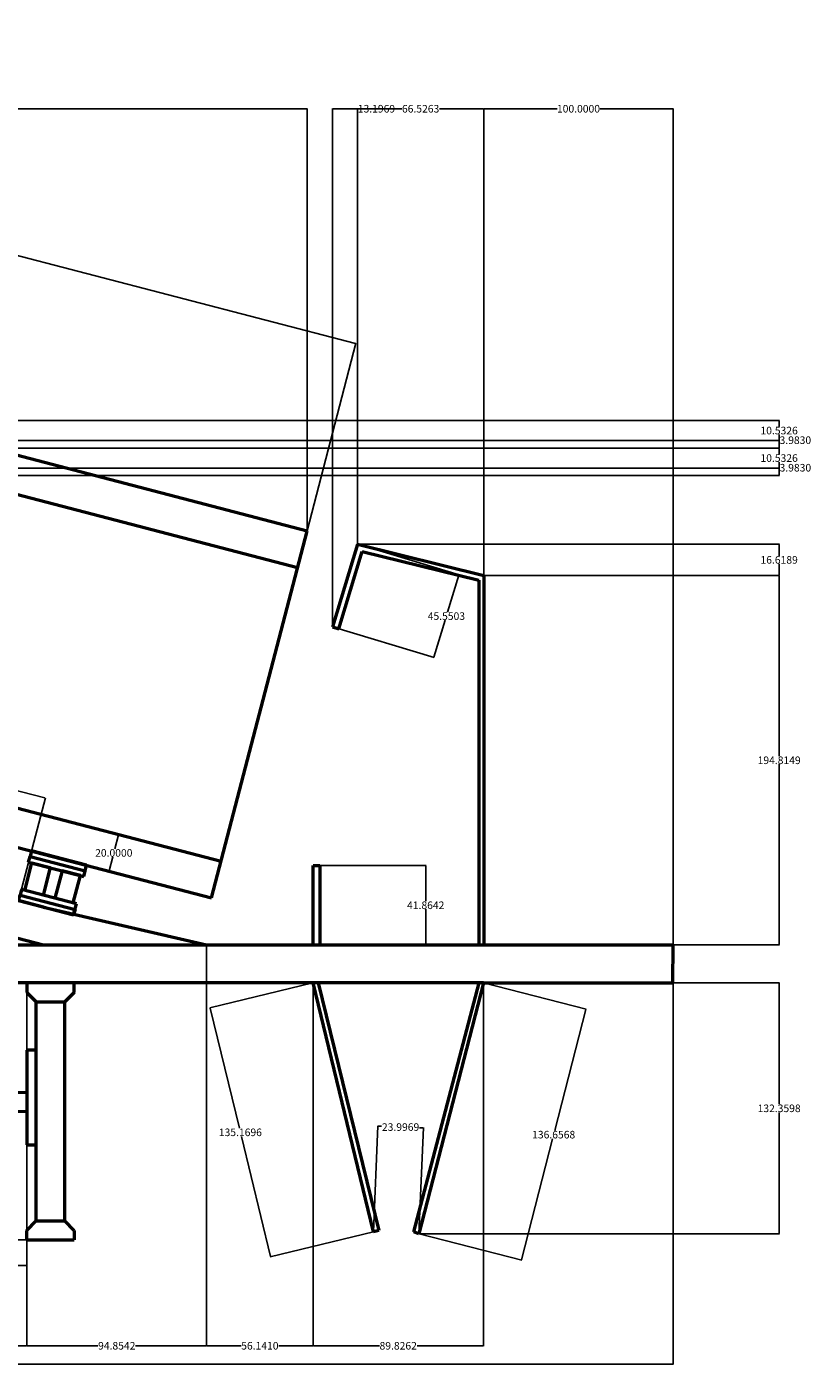
# Model space of a CAD drawing. Units: millimetres. Extents: x -54 to 1187, y -193 to 515.
# Tile 3 of 3: x 773 to 1187, y -193 to 515. Entities that reach past the tile are written whole.
import ezdxf

# ---------------------------------------------------------------- set-up
doc = ezdxf.new("R2010")
doc.units = ezdxf.units.MM
doc.header["$MEASUREMENT"] = 0
doc.layers.add('M-DIMS', color=2, linetype='Continuous', lineweight=25)
doc.layers.add('M-OUTL', color=7, linetype='Continuous', lineweight=50)
doc.styles.get("Standard").update_dxf_attribs({"font": 'arial.ttf'})
doc.dimstyles.get("Standard").update_dxf_attribs({"dimtxt": 4, "dimasz": 0.18, "dimexe": 0.18, "dimexo": 0.0625, "dimgap": 0.09, "dimtad": 0, "dimtih": 1, "dimtoh": 1, "dimdec": 4, "dimzin": 0, "dimdsep": 46, "dimtxsty": 'Standard', "dimcen": 0.09, "dimclrd": 3, "dimclre": 3, "dimclrt": 1, "dimadec": 0, "dimazin": 0, "dimtfac": 1, "dimtdec": 4, "dimtofl": 0, "dimtmove": 0, "dimatfit": 3, "dimfxl": 1, "dimtolj": 1, "dimtzin": 0, "dimarcsym": 0})

# ---------------------------------------------------------------- blocks, each defined once
blk = doc.blocks.new('*D1')
at = {"layer": 'Defpoints', "color": 0, "transparency": 16777216}
for p in [(13.68, 20.33), (1113.76, 20.33), (1113.76, -190.81)]:
    blk.add_point(p, dxfattribs=at)
at = {"layer": 'M-DIMS', "color": 0, "lineweight": -2, "transparency": 16777216}
for p, q in [((13.68, 20.27), (13.68, -190.99)), ((1113.76, 20.27), (1113.76, -190.99)), ((13.86, -190.81), (550.84, -190.81)), ((1113.58, -190.81), (576.6, -190.81))]:
    blk.add_line(p, q, dxfattribs=at)
at = {"layer": 'M-DIMS', "color": 0, "transparency": 16777216}
for points in [[(13.86, -190.78), (13.86, -190.84), (13.68, -190.81)], [(1113.58, -190.78), (1113.58, -190.84), (1113.76, -190.81)]]:
    blk.add_solid(points, dxfattribs=at)
at = {"layer": 'M-DIMS', "color": 0, "transparency": 16777216, "insert": (563.72, -190.81), "char_height": 4, "attachment_point": 5}
blk.add_mtext('\\A1;1100.0835', dxfattribs=at)
blk = doc.blocks.new('*D4')
at = {"layer": 'Defpoints', "color": 0, "transparency": 16777216}
for p in [(643.49, -51.86), (772.88, -51.86), (772.88, -138.82)]:
    blk.add_point(p, dxfattribs=at)
at = {"layer": 'M-DIMS', "color": 0, "lineweight": -2, "transparency": 16777216}
for p, q in [((643.49, -51.92), (643.49, -139)), ((772.88, -51.92), (772.88, -139)), ((643.67, -138.82), (696.87, -138.82)), ((772.7, -138.82), (719.5, -138.82))]:
    blk.add_line(p, q, dxfattribs=at)
at = {"layer": 'M-DIMS', "color": 0, "transparency": 16777216}
for points in [[(643.67, -138.79), (643.67, -138.85), (643.49, -138.82)], [(772.7, -138.79), (772.7, -138.85), (772.88, -138.82)]]:
    blk.add_solid(points, dxfattribs=at)
at = {"layer": 'M-DIMS', "color": 0, "transparency": 16777216, "insert": (708.19, -138.82), "char_height": 4, "attachment_point": 5}
blk.add_mtext('\\A1;129.3903', dxfattribs=at)
blk = doc.blocks.new('*D6')
at = {"layer": 'Defpoints', "color": 0, "transparency": 16777216}
for p in [(279.97, 415.58), (946.42, 347.55), (920.66, 248.68)]:
    blk.add_point(p, dxfattribs=at)
at = {"layer": 'M-DIMS', "color": 0, "lineweight": -2, "transparency": 16777216}
for p, q in [((279.99, 415.64), (305.78, 514.63)), ((305.91, 514.41), (617.89, 433.14)), ((946.25, 347.6), (634.26, 428.87)), ((920.68, 248.74), (946.47, 347.73))]:
    blk.add_line(p, q, dxfattribs=at)
at = {"layer": 'M-DIMS', "color": 0, "transparency": 16777216}
for points in [[(305.91, 514.44), (305.9, 514.38), (305.73, 514.46)], [(946.26, 347.63), (946.24, 347.57), (946.42, 347.55)]]:
    blk.add_solid(points, dxfattribs=at)
at = {"layer": 'M-DIMS', "color": 0, "transparency": 16777216, "insert": (626.08, 431.01), "char_height": 4, "attachment_point": 5}
blk.add_mtext('\\A1;662.0724', dxfattribs=at)
blk = doc.blocks.new('ROLLER-BEARING-UNIT')
for p, q in [((5.29, 27.88), (6.05, 30.79)), ((6.81, 33.69), (6.05, 30.79)), ((6.05, 30.79), (35.08, 23.23)), ((35.84, 26.13), (6.81, 33.69)), ((3.24, 12.92), (7.02, 27.44)), ((5.29, 27.88), (34.33, 20.32)), ((7.02, 27.44), (16.7, 24.91)), ((16.7, 24.91), (12.91, 10.4)), ((22.91, 23.3), (19.12, 8.78)), ((32.58, 20.78), (22.91, 23.3)), ((34.33, 20.32), (35.84, 26.13)), ((28.8, 6.26), (32.58, 20.78)), ((0, 7.56), (0.76, 10.47)), ((0, 7.56), (29.03, 0)), ((1.51, 13.37), (0.76, 10.47)), ((0.76, 10.47), (29.79, 2.9)), ((30.54, 5.81), (1.51, 13.37)), ((30.54, 5.81), (28.8, 6.26)), ((29.03, 0), (30.54, 5.81)), ((29.79, 2.9), (29.03, 0))]:
    blk.add_line(p, q)
blk = doc.blocks.new('FLANGE-PLATE')
for p, q in [((0, 50), (0, 0)), ((5, 50), (0, 50)), ((5, 0), (5, 50)), ((0, 0), (5, 0))]:
    blk.add_line(p, q)
blk = doc.blocks.new('*D13')
at = {"layer": 'Defpoints', "color": 0, "transparency": 16777216}
for p in [(-42.17, 415.58), (279.97, 415.58), (772.86, -125.25)]:
    blk.add_point(p, dxfattribs=at)
at = {"layer": 'M-DIMS', "color": 3, "lineweight": -2, "transparency": 16777216}
for p, q in [((279.91, 415.58), (-42.35, 415.58)), ((-42.17, 415.4), (-42.17, 147.3)), ((-42.17, -125.07), (-42.17, 143.03)), ((772.79, -125.25), (-42.35, -125.25))]:
    blk.add_line(p, q, dxfattribs=at)
at = {"layer": 'M-DIMS', "color": 3, "transparency": 16777216}
for points in [[(-42.2, 415.4), (-42.14, 415.4), (-42.17, 415.58)], [(-42.2, -125.07), (-42.14, -125.07), (-42.17, -125.25)]]:
    blk.add_solid(points, dxfattribs=at)
at = {"layer": 'M-DIMS', "color": 1, "transparency": 16777216, "insert": (-42.17, 145.16), "char_height": 4, "attachment_point": 5}
blk.add_mtext('\\A1;540.8329', dxfattribs=at)
blk = doc.blocks.new('*D18')
at = {"layer": 'Defpoints', "color": 0, "transparency": 16777216}
for p in [(618.49, 10.33), (772.86, 10.33), (772.86, -181.1)]:
    blk.add_point(p, dxfattribs=at)
at = {"layer": 'M-DIMS', "color": 3, "lineweight": -2, "transparency": 16777216}
for p, q in [((618.49, 10.27), (618.49, -181.28)), ((772.86, 10.27), (772.86, -181.28)), ((618.67, -181.1), (684.38, -181.1)), ((772.68, -181.1), (706.97, -181.1))]:
    blk.add_line(p, q, dxfattribs=at)
at = {"layer": 'M-DIMS', "color": 3, "transparency": 16777216}
for points in [[(618.67, -181.07), (618.67, -181.13), (618.49, -181.1)], [(772.68, -181.07), (772.68, -181.13), (772.86, -181.1)]]:
    blk.add_solid(points, dxfattribs=at)
at = {"layer": 'M-DIMS', "color": 1, "transparency": 16777216, "insert": (695.67, -181.1), "char_height": 4, "attachment_point": 5}
blk.add_mtext('\\A1;154.3662', dxfattribs=at)
blk = doc.blocks.new('*D19')
at = {"layer": 'Defpoints', "color": 0, "transparency": 16777216}
for p in [(867.71, 30.33), (772.86, 10.33), (867.71, -181.1)]:
    blk.add_point(p, dxfattribs=at)
at = {"layer": 'M-DIMS', "color": 3, "lineweight": -2, "transparency": 16777216}
for p, q in [((867.71, 30.27), (867.71, -181.28)), ((772.86, 10.27), (772.86, -181.28)), ((773.04, -181.1), (810.36, -181.1)), ((867.53, -181.1), (830.21, -181.1))]:
    blk.add_line(p, q, dxfattribs=at)
at = {"layer": 'M-DIMS', "color": 3, "transparency": 16777216}
for points in [[(773.04, -181.07), (773.04, -181.13), (772.86, -181.1)], [(867.53, -181.07), (867.53, -181.13), (867.71, -181.1)]]:
    blk.add_solid(points, dxfattribs=at)
at = {"layer": 'M-DIMS', "color": 1, "transparency": 16777216, "insert": (820.28, -181.1), "char_height": 4, "attachment_point": 5}
blk.add_mtext('\\A1;94.8542', dxfattribs=at)
blk = doc.blocks.new('*D20')
at = {"layer": 'Defpoints', "color": 0, "transparency": 16777216}
for p in [(867.71, 30.33), (923.85, 10.33), (923.85, -181.1)]:
    blk.add_point(p, dxfattribs=at)
at = {"layer": 'M-DIMS', "color": 3, "lineweight": -2, "transparency": 16777216}
for p, q in [((867.71, 30.27), (867.71, -181.28)), ((923.85, 10.27), (923.85, -181.28)), ((867.89, -181.1), (885.84, -181.1)), ((923.67, -181.1), (905.72, -181.1))]:
    blk.add_line(p, q, dxfattribs=at)
at = {"layer": 'M-DIMS', "color": 3, "transparency": 16777216}
for points in [[(867.89, -181.07), (867.89, -181.13), (867.71, -181.1)], [(923.67, -181.07), (923.67, -181.13), (923.85, -181.1)]]:
    blk.add_solid(points, dxfattribs=at)
at = {"layer": 'M-DIMS', "color": 1, "transparency": 16777216, "insert": (895.78, -181.1), "char_height": 4, "attachment_point": 5}
blk.add_mtext('\\A1;56.1410', dxfattribs=at)
blk = doc.blocks.new('*D21')
at = {"layer": 'Defpoints', "color": 0, "transparency": 16777216}
for p in [(923.85, 10.33), (1013.68, 10.33), (1013.68, -181.1)]:
    blk.add_point(p, dxfattribs=at)
at = {"layer": 'M-DIMS', "color": 3, "lineweight": -2, "transparency": 16777216}
for p, q in [((923.85, 10.27), (923.85, -181.28)), ((1013.68, 10.27), (1013.68, -181.28)), ((924.03, -181.1), (958.84, -181.1)), ((1013.5, -181.1), (978.69, -181.1))]:
    blk.add_line(p, q, dxfattribs=at)
at = {"layer": 'M-DIMS', "color": 3, "transparency": 16777216}
for points in [[(924.03, -181.07), (924.03, -181.13), (923.85, -181.1)], [(1013.5, -181.07), (1013.5, -181.13), (1013.68, -181.1)]]:
    blk.add_solid(points, dxfattribs=at)
at = {"layer": 'M-DIMS', "color": 1, "transparency": 16777216, "insert": (968.76, -181.1), "char_height": 4, "attachment_point": 5}
blk.add_mtext('\\A1;89.8262', dxfattribs=at)
blk = doc.blocks.new('*D22')
at = {"layer": 'Defpoints', "color": 0, "transparency": 16777216}
for p in [(1113.85, 471.43), (1013.85, 30.33), (1113.85, 30.33)]:
    blk.add_point(p, dxfattribs=at)
at = {"layer": 'M-DIMS', "color": 3, "lineweight": -2, "transparency": 16777216}
for p, q in [((1013.85, 30.39), (1013.85, 471.61)), ((1014.03, 471.43), (1052.54, 471.43)), ((1113.67, 471.43), (1075.15, 471.43)), ((1113.85, 30.39), (1113.85, 471.61))]:
    blk.add_line(p, q, dxfattribs=at)
at = {"layer": 'M-DIMS', "color": 3, "transparency": 16777216}
for points in [[(1014.03, 471.46), (1014.03, 471.4), (1013.85, 471.43)], [(1113.67, 471.46), (1113.67, 471.4), (1113.85, 471.43)]]:
    blk.add_solid(points, dxfattribs=at)
at = {"layer": 'M-DIMS', "color": 1, "transparency": 16777216, "insert": (1063.85, 471.43), "char_height": 4, "attachment_point": 5}
blk.add_mtext('\\A1;100.0000', dxfattribs=at)
blk = doc.blocks.new('*D23')
at = {"layer": 'Defpoints', "color": 0, "transparency": 16777216}
for p in [(923.85, 10.33), (869.57, -2.83), (955.7, -121.03)]:
    blk.add_point(p, dxfattribs=at)
at = {"layer": 'M-DIMS', "color": 3, "lineweight": -2, "transparency": 16777216}
for p, q in [((923.79, 10.32), (869.4, -2.87)), ((869.62, -3), (884.98, -66.38)), ((901.38, -134.02), (886.02, -70.64)), ((955.64, -121.05), (901.25, -134.24))]:
    blk.add_line(p, q, dxfattribs=at)
at = {"layer": 'M-DIMS', "color": 3, "transparency": 16777216}
for points in [[(869.65, -3), (869.59, -3.01), (869.57, -2.83)], [(901.41, -134.01), (901.35, -134.03), (901.43, -134.19)]]:
    blk.add_solid(points, dxfattribs=at)
at = {"layer": 'M-DIMS', "color": 1, "transparency": 16777216, "insert": (885.5, -68.51), "char_height": 4, "attachment_point": 5}
blk.add_mtext('\\A1;135.1696', dxfattribs=at)
blk = doc.blocks.new('*D24')
at = {"layer": 'Defpoints', "color": 0, "transparency": 16777216}
for p in [(1013.68, 10.33), (979.68, -122.03), (1033.77, -135.92)]:
    blk.add_point(p, dxfattribs=at)
at = {"layer": 'M-DIMS', "color": 3, "lineweight": -2, "transparency": 16777216}
for p, q in [((1013.74, 10.32), (1067.95, -3.61)), ((1067.73, -3.74), (1051.32, -67.61)), ((1033.82, -135.75), (1050.22, -71.88)), ((979.74, -122.04), (1033.95, -135.97))]:
    blk.add_line(p, q, dxfattribs=at)
at = {"layer": 'M-DIMS', "color": 3, "transparency": 16777216}
for points in [[(1067.7, -3.73), (1067.76, -3.75), (1067.77, -3.56)], [(1033.79, -135.74), (1033.85, -135.76), (1033.77, -135.92)]]:
    blk.add_solid(points, dxfattribs=at)
at = {"layer": 'M-DIMS', "color": 1, "transparency": 16777216, "insert": (1050.77, -69.74), "char_height": 4, "attachment_point": 5}
blk.add_mtext('\\A1;136.6568', dxfattribs=at)
blk = doc.blocks.new('*D25')
at = {"layer": 'Defpoints', "color": 0, "transparency": 16777216}
for p in [(982, -66.23), (955.7, -121.03), (979.68, -122.03)]:
    blk.add_point(p, dxfattribs=at)
at = {"layer": 'M-DIMS', "color": 3, "lineweight": -2, "transparency": 16777216}
for p, q in [((955.71, -120.97), (958.03, -65.05)), ((958.2, -65.24), (960.02, -65.31)), ((979.68, -121.97), (982.01, -66.05)), ((981.82, -66.22), (979.99, -66.14))]:
    blk.add_line(p, q, dxfattribs=at)
at = {"layer": 'M-DIMS', "color": 3, "transparency": 16777216}
for points in [[(958.2, -65.21), (958.2, -65.27), (958.02, -65.23)], [(981.82, -66.19), (981.82, -66.25), (982, -66.23)]]:
    blk.add_solid(points, dxfattribs=at)
at = {"layer": 'M-DIMS', "color": 1, "transparency": 16777216, "insert": (970.01, -65.73), "char_height": 4, "attachment_point": 5}
blk.add_mtext('\\A1;23.9969', dxfattribs=at)
blk = doc.blocks.new('*D29')
at = {"layer": 'Defpoints', "color": 0, "transparency": 16777216}
for p in [(920.66, 471.43), (279.97, 415.58), (920.66, 248.68)]:
    blk.add_point(p, dxfattribs=at)
at = {"layer": 'M-DIMS', "color": 3, "lineweight": -2, "transparency": 16777216}
for p, q in [((279.97, 415.64), (279.97, 471.61)), ((280.15, 471.43), (588.81, 471.43)), ((920.48, 471.43), (611.83, 471.43)), ((920.66, 248.74), (920.66, 471.61))]:
    blk.add_line(p, q, dxfattribs=at)
at = {"layer": 'M-DIMS', "color": 3, "transparency": 16777216}
for points in [[(280.15, 471.46), (280.15, 471.4), (279.97, 471.43)], [(920.48, 471.46), (920.48, 471.4), (920.66, 471.43)]]:
    blk.add_solid(points, dxfattribs=at)
at = {"layer": 'M-DIMS', "color": 1, "transparency": 16777216, "insert": (600.32, 471.43), "char_height": 4, "attachment_point": 5}
blk.add_mtext('\\A1;640.6893', dxfattribs=at)
blk = doc.blocks.new('*D32')
at = {"layer": 'Defpoints', "color": 0, "transparency": 16777216}
for p in [(821.24, 88.57), (875.29, 74.49), (870.25, 55.14)]:
    blk.add_point(p, dxfattribs=at)
at = {"layer": 'M-DIMS', "color": 3, "lineweight": -2, "transparency": 16777216}
for p, q in [((821.2, 88.4), (819.28, 81.03)), ((875.23, 74.51), (821.07, 88.62)), ((816.24, 69.39), (818.16, 76.76)), ((870.18, 55.15), (816.03, 69.26))]:
    blk.add_line(p, q, dxfattribs=at)
at = {"layer": 'M-DIMS', "color": 3, "transparency": 16777216}
for points in [[(821.17, 88.4), (821.22, 88.39), (821.24, 88.57)], [(816.22, 69.4), (816.27, 69.38), (816.2, 69.22)]]:
    blk.add_solid(points, dxfattribs=at)
at = {"layer": 'M-DIMS', "color": 1, "transparency": 16777216, "insert": (818.72, 78.89), "char_height": 4, "attachment_point": 5}
blk.add_mtext('\\A1;20.0000', dxfattribs=at)
blk = doc.blocks.new('*D35')
at = {"layer": 'Defpoints', "color": 0, "transparency": 16777216}
for p in [(782.59, 107.81), (588.76, 100.59), (768.51, 53.76)]:
    blk.add_point(p, dxfattribs=at)
at = {"layer": 'M-DIMS', "color": 3, "lineweight": -2, "transparency": 16777216}
for p, q in [((588.78, 100.65), (602.89, 154.81)), ((603.02, 154.59), (684.53, 133.36)), ((782.41, 107.86), (700.9, 129.09)), ((768.52, 53.82), (782.63, 107.98))]:
    blk.add_line(p, q, dxfattribs=at)
at = {"layer": 'M-DIMS', "color": 3, "transparency": 16777216}
for points in [[(603.02, 154.62), (603.01, 154.56), (602.84, 154.64)], [(782.42, 107.88), (782.41, 107.83), (782.59, 107.81)]]:
    blk.add_solid(points, dxfattribs=at)
at = {"layer": 'M-DIMS', "color": 1, "transparency": 16777216, "insert": (692.71, 131.22), "char_height": 4, "attachment_point": 5}
blk.add_mtext('\\A1;185.7466', dxfattribs=at)
blk = doc.blocks.new('*D40')
at = {"layer": 'Defpoints', "color": 0, "transparency": 16777216}
for p in [(1013.85, 225.15), (1169.7, 225.15), (1013.85, 30.33)]:
    blk.add_point(p, dxfattribs=at)
at = {"layer": 'M-DIMS', "color": 3, "lineweight": -2, "transparency": 16777216}
for p, q in [((1013.91, 225.15), (1169.88, 225.15)), ((1169.7, 224.97), (1169.7, 129.87)), ((1169.7, 30.51), (1169.7, 125.61)), ((1013.91, 30.33), (1169.88, 30.33))]:
    blk.add_line(p, q, dxfattribs=at)
at = {"layer": 'M-DIMS', "color": 3, "transparency": 16777216}
for points in [[(1169.67, 224.97), (1169.73, 224.97), (1169.7, 225.15)], [(1169.67, 30.51), (1169.73, 30.51), (1169.7, 30.33)]]:
    blk.add_solid(points, dxfattribs=at)
at = {"layer": 'M-DIMS', "color": 1, "transparency": 16777216, "insert": (1169.7, 127.74), "char_height": 4, "attachment_point": 5}
blk.add_mtext('\\A1;194.8149', dxfattribs=at)
blk = doc.blocks.new('*D41')
at = {"layer": 'Defpoints', "color": 0, "transparency": 16777216}
for p in [(947.32, 241.76), (1169.7, 241.76), (1013.85, 225.15)]:
    blk.add_point(p, dxfattribs=at)
at = {"layer": 'M-DIMS', "color": 3, "lineweight": -2, "transparency": 16777216}
for p, q in [((947.38, 241.76), (1169.88, 241.76)), ((1169.7, 241.58), (1169.7, 235.59)), ((1169.7, 225.33), (1169.7, 231.32)), ((1013.91, 225.15), (1169.88, 225.15))]:
    blk.add_line(p, q, dxfattribs=at)
at = {"layer": 'M-DIMS', "color": 3, "transparency": 16777216}
for points in [[(1169.67, 241.58), (1169.73, 241.58), (1169.7, 241.76)], [(1169.67, 225.33), (1169.73, 225.33), (1169.7, 225.15)]]:
    blk.add_solid(points, dxfattribs=at)
at = {"layer": 'M-DIMS', "color": 1, "transparency": 16777216, "insert": (1169.7, 233.45), "char_height": 4, "attachment_point": 5}
blk.add_mtext('\\A1;16.6189', dxfattribs=at)
blk = doc.blocks.new('*D42')
at = {"layer": 'Defpoints', "color": 0, "transparency": 16777216}
for p in [(1013.68, 10.33), (979.68, -122.03), (1169.7, -122.03)]:
    blk.add_point(p, dxfattribs=at)
at = {"layer": 'M-DIMS', "color": 3, "lineweight": -2, "transparency": 16777216}
for p, q in [((1013.74, 10.33), (1169.88, 10.33)), ((1169.7, 10.15), (1169.7, -53.72)), ((1169.7, -121.85), (1169.7, -57.98)), ((979.74, -122.03), (1169.88, -122.03))]:
    blk.add_line(p, q, dxfattribs=at)
at = {"layer": 'M-DIMS', "color": 3, "transparency": 16777216}
for points in [[(1169.67, 10.15), (1169.73, 10.15), (1169.7, 10.33)], [(1169.67, -121.85), (1169.73, -121.85), (1169.7, -122.03)]]:
    blk.add_solid(points, dxfattribs=at)
at = {"layer": 'M-DIMS', "color": 1, "transparency": 16777216, "insert": (1169.7, -55.85), "char_height": 4, "attachment_point": 5}
blk.add_mtext('\\A1;132.3598', dxfattribs=at)
blk = doc.blocks.new('*D43')
at = {"layer": 'Defpoints', "color": 0, "transparency": 16777216}
for p in [(1013.85, 471.43), (947.32, 241.76), (1013.85, 225.15)]:
    blk.add_point(p, dxfattribs=at)
at = {"layer": 'M-DIMS', "color": 3, "lineweight": -2, "transparency": 16777216}
for p, q in [((947.32, 241.83), (947.32, 471.61)), ((947.5, 471.43), (970.62, 471.43)), ((1013.67, 471.43), (990.54, 471.43)), ((1013.85, 225.21), (1013.85, 471.61))]:
    blk.add_line(p, q, dxfattribs=at)
at = {"layer": 'M-DIMS', "color": 3, "transparency": 16777216}
for points in [[(947.5, 471.46), (947.5, 471.4), (947.32, 471.43)], [(1013.67, 471.46), (1013.67, 471.4), (1013.85, 471.43)]]:
    blk.add_solid(points, dxfattribs=at)
at = {"layer": 'M-DIMS', "color": 1, "transparency": 16777216, "insert": (980.58, 471.43), "char_height": 4, "attachment_point": 5}
blk.add_mtext('\\A1;66.5263', dxfattribs=at)
blk = doc.blocks.new('*D44')
at = {"layer": 'Defpoints', "color": 0, "transparency": 16777216}
for p in [(947.32, 471.43), (947.32, 241.76), (934.12, 198.17)]:
    blk.add_point(p, dxfattribs=at)
at = {"layer": 'M-DIMS', "color": 3, "lineweight": -2, "transparency": 16777216}
for p, q in [((934.12, 198.23), (934.12, 471.61)), ((934.3, 471.43), (947.14, 471.43)), ((947.32, 241.83), (947.32, 471.61)), ((947.32, 471.43), (947.5, 471.43))]:
    blk.add_line(p, q, dxfattribs=at)
at = {"layer": 'M-DIMS', "color": 3, "transparency": 16777216}
for points in [[(934.3, 471.46), (934.3, 471.4), (934.12, 471.43)], [(947.14, 471.46), (947.14, 471.4), (947.32, 471.43)]]:
    blk.add_solid(points, dxfattribs=at)
at = {"layer": 'M-DIMS', "color": 1, "transparency": 16777216, "insert": (957.26, 471.43), "char_height": 4, "attachment_point": 5}
blk.add_mtext('\\A1;13.1969', dxfattribs=at)
blk = doc.blocks.new('*D45')
at = {"layer": 'Defpoints', "color": 0, "transparency": 16777216}
for p in [(947.32, 241.76), (934.12, 198.17), (987.58, 181.99)]:
    blk.add_point(p, dxfattribs=at)
at = {"layer": 'M-DIMS', "color": 3, "lineweight": -2, "transparency": 16777216}
for p, q in [((947.38, 241.75), (1000.95, 225.53)), ((1000.72, 225.41), (994.82, 205.92)), ((987.63, 182.16), (993.53, 201.65)), ((934.18, 198.15), (987.75, 181.93))]:
    blk.add_line(p, q, dxfattribs=at)
at = {"layer": 'M-DIMS', "color": 3, "transparency": 16777216}
for points in [[(1000.69, 225.42), (1000.75, 225.4), (1000.77, 225.58)], [(987.6, 182.17), (987.66, 182.15), (987.58, 181.99)]]:
    blk.add_solid(points, dxfattribs=at)
at = {"layer": 'M-DIMS', "color": 1, "transparency": 16777216, "insert": (994.17, 203.79), "char_height": 4, "attachment_point": 5}
blk.add_mtext('\\A1;45.5503', dxfattribs=at)
blk = doc.blocks.new('*D46')
at = {"layer": 'Defpoints', "color": 0, "transparency": 16777216}
for p in [(927.42, 72.19), (927.42, 30.33), (983.27, 30.33)]:
    blk.add_point(p, dxfattribs=at)
at = {"layer": 'M-DIMS', "color": 3, "lineweight": -2, "transparency": 16777216}
for p, q in [((927.48, 72.19), (983.45, 72.19)), ((983.27, 72.01), (983.27, 53.39)), ((983.27, 30.51), (983.27, 49.13)), ((927.48, 30.33), (983.45, 30.33))]:
    blk.add_line(p, q, dxfattribs=at)
at = {"layer": 'M-DIMS', "color": 3, "transparency": 16777216}
for points in [[(983.24, 72.01), (983.3, 72.01), (983.27, 72.19)], [(983.24, 30.51), (983.3, 30.51), (983.27, 30.33)]]:
    blk.add_solid(points, dxfattribs=at)
at = {"layer": 'M-DIMS', "color": 1, "transparency": 16777216, "insert": (983.27, 51.26), "char_height": 4, "attachment_point": 5}
blk.add_mtext('\\A1;41.8642', dxfattribs=at)
blk = doc.blocks.new('*D51')
at = {"layer": 'Defpoints', "color": 0, "transparency": 16777216}
for p in [(352.28, 277.91), (366.74, 281.89), (1169.7, 281.89)]:
    blk.add_point(p, dxfattribs=at)
at = {"layer": 'M-DIMS', "color": 3, "lineweight": -2, "transparency": 16777216}
for p, q in [((352.34, 277.91), (1169.88, 277.91)), ((366.8, 281.89), (1169.88, 281.89)), ((1169.7, 281.89), (1169.7, 282.07)), ((1169.7, 282.07), (1169.88, 282.07)), ((1169.7, 278.09), (1169.7, 281.71))]:
    blk.add_line(p, q, dxfattribs=at)
at = {"layer": 'M-DIMS', "color": 3, "transparency": 16777216}
for points in [[(1169.67, 281.71), (1169.73, 281.71), (1169.7, 281.89)], [(1169.67, 278.09), (1169.73, 278.09), (1169.7, 277.91)]]:
    blk.add_solid(points, dxfattribs=at)
at = {"layer": 'M-DIMS', "color": 1, "transparency": 16777216, "insert": (1178.26, 282.07), "char_height": 4, "attachment_point": 5}
blk.add_mtext('\\A1;3.9830', dxfattribs=at)
blk = doc.blocks.new('*D52')
at = {"layer": 'Defpoints', "color": 0, "transparency": 16777216}
for p in [(356.06, 292.42), (1169.7, 292.42), (366.74, 281.89)]:
    blk.add_point(p, dxfattribs=at)
at = {"layer": 'M-DIMS', "color": 3, "lineweight": -2, "transparency": 16777216}
for p, q in [((356.12, 292.42), (1169.88, 292.42)), ((1169.7, 292.24), (1169.7, 289.29)), ((1169.7, 282.07), (1169.7, 285.02)), ((366.8, 281.89), (1169.88, 281.89))]:
    blk.add_line(p, q, dxfattribs=at)
at = {"layer": 'M-DIMS', "color": 3, "transparency": 16777216}
for points in [[(1169.67, 292.24), (1169.73, 292.24), (1169.7, 292.42)], [(1169.67, 282.07), (1169.73, 282.07), (1169.7, 281.89)]]:
    blk.add_solid(points, dxfattribs=at)
at = {"layer": 'M-DIMS', "color": 1, "transparency": 16777216, "insert": (1169.7, 287.16), "char_height": 4, "attachment_point": 5}
blk.add_mtext('\\A1;10.5326', dxfattribs=at)
blk = doc.blocks.new('*D53')
at = {"layer": 'Defpoints', "color": 0, "transparency": 16777216}
for p in [(356.06, 292.42), (370.52, 296.41), (1169.7, 296.41)]:
    blk.add_point(p, dxfattribs=at)
at = {"layer": 'M-DIMS', "color": 3, "lineweight": -2, "transparency": 16777216}
for p, q in [((356.12, 292.42), (1169.88, 292.42)), ((370.58, 296.41), (1169.88, 296.41)), ((1169.7, 296.41), (1169.7, 296.59)), ((1169.7, 296.59), (1169.88, 296.59)), ((1169.7, 292.6), (1169.7, 296.23))]:
    blk.add_line(p, q, dxfattribs=at)
at = {"layer": 'M-DIMS', "color": 3, "transparency": 16777216}
for points in [[(1169.67, 296.23), (1169.73, 296.23), (1169.7, 296.41)], [(1169.67, 292.6), (1169.73, 292.6), (1169.7, 292.42)]]:
    blk.add_solid(points, dxfattribs=at)
at = {"layer": 'M-DIMS', "color": 1, "transparency": 16777216, "insert": (1178.26, 296.59), "char_height": 4, "attachment_point": 5}
blk.add_mtext('\\A1;3.9830', dxfattribs=at)
blk = doc.blocks.new('*D54')
at = {"layer": 'Defpoints', "color": 0, "transparency": 16777216}
for p in [(359.84, 306.94), (1169.7, 306.94), (370.52, 296.41)]:
    blk.add_point(p, dxfattribs=at)
at = {"layer": 'M-DIMS', "color": 3, "lineweight": -2, "transparency": 16777216}
for p, q in [((359.9, 306.94), (1169.88, 306.94)), ((1169.7, 306.76), (1169.7, 303.81)), ((1169.7, 296.59), (1169.7, 299.54)), ((370.58, 296.41), (1169.88, 296.41))]:
    blk.add_line(p, q, dxfattribs=at)
at = {"layer": 'M-DIMS', "color": 3, "transparency": 16777216}
for points in [[(1169.67, 306.76), (1169.73, 306.76), (1169.7, 306.94)], [(1169.67, 296.59), (1169.73, 296.59), (1169.7, 296.41)]]:
    blk.add_solid(points, dxfattribs=at)
at = {"layer": 'M-DIMS', "color": 1, "transparency": 16777216, "insert": (1169.7, 301.67), "char_height": 4, "attachment_point": 5}
blk.add_mtext('\\A1;10.5326', dxfattribs=at)

msp = doc.modelspace()

# ---------------------------------------------------------------- linework, layer by layer
at = {"layer": 'M-OUTL'}
for p, q in [((920.66417, 248.67693), (279.97484, 415.5813)), ((915.62229, 229.32287), (274.93296, 396.22724)), ((870.2454, 55.13637), (920.66417, 248.67693)), ((234.59795, 241.3948), (875.28728, 74.49042)), ((947.31877, 241.76432), (934.12187, 198.16761)), ((947.31877, 241.76432), (946.40031, 238.73016)), ((947.31877, 241.76432), (1013.84504, 225.14543)), ((947.31877, 241.76432), (947.31877, 241.76432)), ((937.45204, 197.15955), (949.66538, 237.92258)), ((949.66538, 237.92258), (1011.30715, 222.67625)), ((229.55607, 222.04074), (870.2454, 55.13637)), ((1011.30715, 222.67625), (1011.30715, 30.33057)), ((1013.84504, 225.14543), (1013.84504, 30.33057)), ((781.59027, 50.33057), (222.74954, 195.91276)), ((934.12187, 198.16761), (937.45204, 197.15955)), ((222.74954, 175.91276), (781.59027, 30.33057)), ((923.92724, 30.33057), (923.92724, 72.19475)), ((923.92724, 72.19475), (927.41655, 72.19475)), ((927.41655, 72.19475), (927.41655, 30.33057)), ((781.59027, 50.33057), (867.7109, 30.33057)), ((13.67803, 30.33057), (1013.67803, 30.33057)), ((1013.84504, 30.33057), (1113.84504, 30.33057)), ((1113.67803, 10.33057), (1113.84504, 30.33057)), ((1013.67803, 10.33057), (13.67803, 10.33057)), ((772.85666, 10.33057), (772.85666, 5.33057)), ((797.85666, 5.33057), (797.85666, 10.33057)), ((955.70241, -121.03288), (923.85187, 10.33057)), ((926.61434, 10.33057), (958.56516, -120.36178)), ((977.02071, -121.04027), (1011.43769, 10.33057)), ((1013.67803, 10.33057), (979.67865, -122.02926)), ((1013.67803, 10.33057), (1113.67803, 10.33057)), ((772.85666, 5.33057), (777.85666, 0.33057)), ((777.85666, -115.25163), (777.85666, 0.33057)), ((777.85666, 0.33057), (792.85666, 0.33057)), ((797.85666, 5.33057), (792.85666, 0.33057)), ((792.85666, -115.25163), (792.85666, 0.33057)), ((643.4905, -46.87914), (772.85666, -47.43885)), ((777.85666, -47.46049), (777.8783, -47.46058)), ((643.4905, -56.87924), (772.85666, -57.43895)), ((772.85666, -120.25163), (777.85666, -115.25163)), ((772.85666, -125.25163), (772.85666, -120.25163)), ((777.85666, -115.25163), (792.85666, -115.25163)), ((797.85666, -120.25163), (792.85666, -115.25163)), ((797.85666, -120.25163), (797.85666, -125.25163)), ((958.56516, -120.36178), (955.70241, -121.03288)), ((772.85666, -125.25163), (797.85666, -125.25163)), ((979.67865, -122.02926), (977.02071, -121.04027))]:
    msp.add_line(p, q, dxfattribs=at)

# ---------------------------------------------------------------- block references
msp.add_blockref('ROLLER-BEARING-UNIT', (768.50893, 46.20096), dxfattribs=at)
at = {"layer": 'M-OUTL', "rotation": 180}
msp.add_blockref('FLANGE-PLATE', (777.85683, -25.13188), dxfattribs=at)

# ---------------------------------------------------------------- dimensions: what is measured, and where the dimension line sits
at = {"layer": 'M-DIMS'}
dim = msp.add_aligned_dim(p1=(279.97484, 415.5813), p2=(920.66417, 248.67693), distance=102.17685, dimstyle='Standard', override={"dimclrd": 0, "dimclre": 0, "dimclrt": 0}, dxfattribs=at)
dim.commit()
dim.dimension.update_dxf_attribs({"geometry": '*D6', "text_midpoint": (626.07766, 431.00594)})
for base, p1, p2, override, picture, middle in [((920.66417, 471.4313), (279.97484, 415.5813), (920.66417, 248.67693), {"dimdec": 4, "dimlfac": 1, "dimrnd": 0, "dimzin": 0, "dimdsep": 46, "dimlunit": 2}, '*D29', (600.3195, 471.4313)), ((947.31877, 471.4313), (934.12187, 198.16761), (947.31877, 241.76432), {"dimdec": 4, "dimlfac": 1, "dimrnd": 0, "dimzin": 0, "dimdsep": 46, "dimlunit": 2}, '*D44', (957.26135, 471.4313)), ((1013.84504, 471.4313), (947.31877, 241.76432), (1013.84504, 225.14543), {"dimdec": 4, "dimlfac": 1, "dimrnd": 0, "dimzin": 0, "dimdsep": 46, "dimlunit": 2}, '*D43', (980.5819, 471.4313)), ((1113.84504, 471.4313), (1013.84504, 30.33057), (1113.84504, 30.33057), {"dimdec": 4, "dimlfac": 1, "dimrnd": 0, "dimzin": 0, "dimdsep": 46, "dimlunit": 2}, '*D22', (1063.84504, 471.4313)), ((867.7109, -181.10163), (772.85666, 10.33057), (867.7109, 30.33057), {"dimdec": 4, "dimlfac": 1, "dimrnd": 0, "dimzin": 0, "dimdsep": 46, "dimlunit": 2}, '*D19', (820.28378, -181.10163)), ((923.85187, -181.10163), (867.7109, 30.33057), (923.85187, 10.33057), {"dimdec": 4, "dimlfac": 1, "dimrnd": 0, "dimzin": 0, "dimdsep": 46, "dimlunit": 2}, '*D20', (895.78139, -181.10163)), ((1113.76153, -190.8134), (13.67803, 20.33057), (1113.76153, 20.33057), {"dimclrd": 0, "dimclre": 0, "dimclrt": 0}, '*D1', (563.71978, -190.8134)), ((772.85666, -181.10163), (618.4905, 10.33057), (772.85666, 10.33057), {"dimdec": 4, "dimlfac": 1, "dimrnd": 0, "dimzin": 0, "dimdsep": 46, "dimlunit": 2}, '*D18', (695.67358, -181.10163)), ((1013.67803, -181.10163), (923.85187, 10.33057), (1013.67803, 10.33057), {"dimdec": 4, "dimlfac": 1, "dimrnd": 0, "dimzin": 0, "dimdsep": 46, "dimlunit": 2}, '*D21', (968.76495, -181.10163)), ((772.88081, -138.82183), (643.4905, -51.85756), (772.88081, -51.85756), {"dimclrd": 0, "dimclre": 0, "dimclrt": 0}, '*D4', (708.18566, -138.82183))]:
    dim = msp.add_linear_dim(base=base, p1=p1, p2=p2, dimstyle='Standard', override=override, dxfattribs=at)
    dim.commit()
    dim.dimension.update_dxf_attribs({"geometry": picture, "text_midpoint": middle})
for base, p1, p2, angle, picture, middle in [((-42.17197, 415.5813), (772.85666, -125.25163), (279.97484, 415.5813), 90, '*D13', (-42.17197, 145.16483)), ((1169.69504, 306.939), (370.5199, 296.40643), (359.83977, 306.939), 90, '*D54', (1169.69504, 301.67272)), ((1169.69504, 296.40643), (356.05837, 292.42346), (370.5199, 296.40643), 90, '*D53', (1178.25972, 296.58643)), ((1169.69504, 292.42346), (366.73849, 281.89089), (356.05837, 292.42346), 90, '*D52', (1169.69504, 287.15717)), ((1169.69504, 281.89089), (352.27696, 277.90792), (366.73849, 281.89089), 90, '*D51', (1178.25972, 282.07089)), ((987.57652, 181.98668), (947.31877, 241.76432), (934.12187, 198.16761), 253.1587286, '*D45', (994.17497, 203.78503)), ((1169.69504, 241.76432), (1013.84504, 225.14543), (947.31877, 241.76432), 90, '*D41', (1169.69504, 233.45487)), ((1169.69504, 225.14543), (1013.84504, 30.33057), (1013.84504, 225.14543), 90, '*D40', (1169.69504, 127.738)), ((782.58839, 107.81036), (588.76147, 100.58973), (768.50895, 53.76416), 345.39855107, '*D35', (692.71465, 131.22315)), ((821.24108, 88.56986), (870.2454, 55.13637), (875.28728, 74.49042), 75.39855107, '*D32', (818.72014, 78.89284)), ((983.26656, 30.33057), (927.41655, 72.19475), (927.41655, 30.33057), 270, '*D46', (983.26656, 51.26266)), ((869.5745, -2.82959), (955.70241, -121.03288), (923.85187, 10.33057), 103.62899432, '*D23', (885.49977, -68.51131)), ((1033.77252, -135.9244), (1013.67803, 10.33057), (979.67865, -122.02926), 255.59384661, '*D24', (1050.77221, -69.74449)), ((1169.69504, -122.02926), (1013.67803, 10.33057), (979.67865, -122.02926), 90, '*D42', (1169.69504, -55.84935)), ((981.99761, -66.22742), (955.70241, -121.03288), (979.67865, -122.02926), 357.62032302, '*D25', (970.00949, -65.72923))]:
    dim = msp.add_linear_dim(base=base, p1=p1, p2=p2, angle=angle, dimstyle='Standard', override={"dimdec": 4, "dimlfac": 1, "dimrnd": 0, "dimzin": 0, "dimdsep": 46, "dimlunit": 2}, dxfattribs=at)
    dim.commit()
    dim.dimension.update_dxf_attribs({"geometry": picture, "text_midpoint": middle})

doc.saveas('drawing.dxf')
